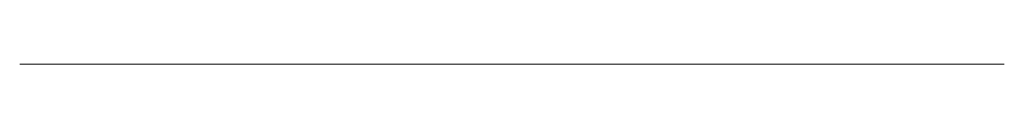
# Model space of a CAD drawing. Units: millimetres. Extents: x 412 to 562, y 0 to 0.
import ezdxf

# ---------------------------------------------------------------- set-up
doc = ezdxf.new("R2010")
doc.units = ezdxf.units.MM
doc.layers.add('M-CONS', color=8, linetype='Continuous', lineweight=13)

msp = doc.modelspace()

# ---------------------------------------------------------------- linework, layer by layer
at = {"layer": 'M-CONS', "extrusion": (0, -1, 0)}
for p, q in [((412.43, 0, 107.02), (412.43, 0, 115.59)), ((412.43, 0, 158.46), (412.43, 0, 167.02)), ((412.43, 0, 158.46), (412.43, 0, 115.59)), ((562.43, 0, 107.02), (527.43, 0, 107.02)), ((562.43, 0, 167.02), (562.43, 0, 107.02))]:
    msp.add_line(p, q, dxfattribs=at)
for centre, radius, start, end in [((469.93, -31.52), 150, 67.4597, 112.5403), ((487.43, 3.39), 180, 65.3757, 114.6243)]:
    msp.add_arc(centre, radius, start, end, dxfattribs=at)

doc.saveas('drawing.dxf')
